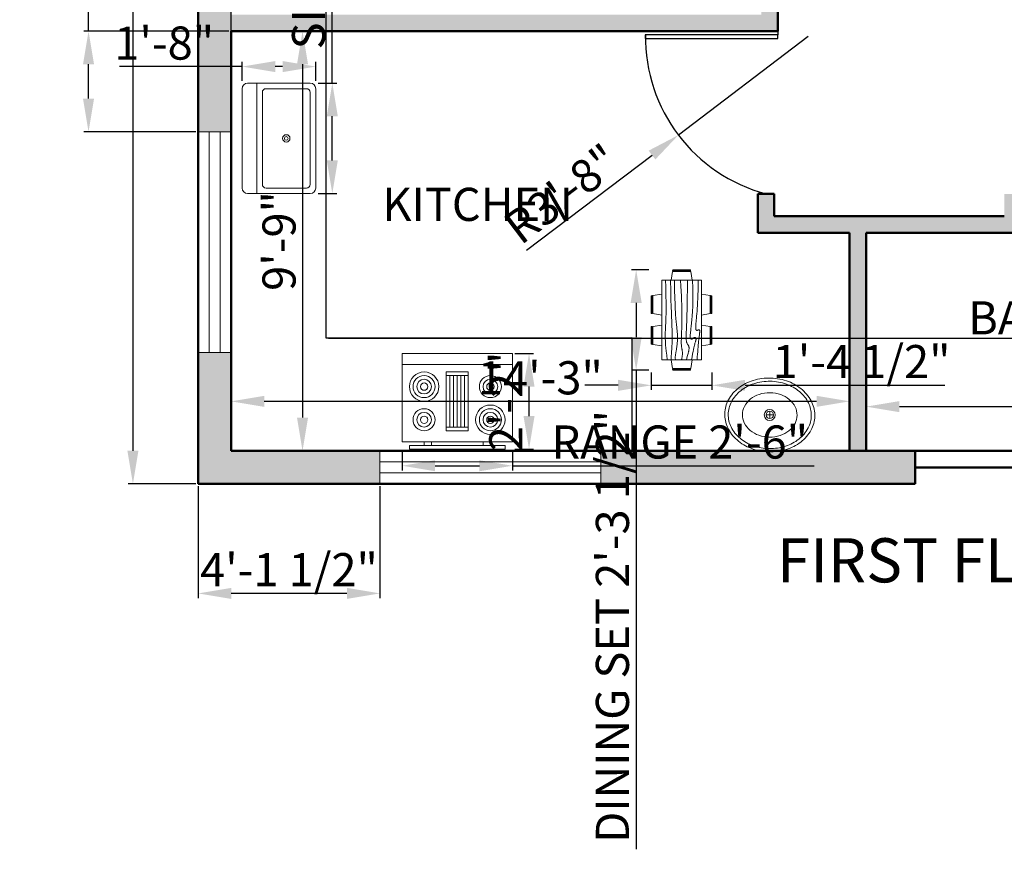
# Model space of a CAD drawing. Units: inches. Extents: x 875413 to 876020, y 447446 to 448210.
# Tile 1 of 8: x 875413 to 875681, y 447446 to 447671. Entities that reach past the tile are written whole.
import ezdxf

# ---------------------------------------------------------------- set-up
doc = ezdxf.new("R2010")
doc.units = ezdxf.units.IN
for name, color, linetype, lineweight in [('A-ANNO-DIMS', 2, 'Continuous', 13), ('A-ANNO-TEXT', 7, 'Continuous', 35), ('A-AREA-IDEN', 7, 'Continuous', 25), ('A-DOOR', 3, 'Continuous', 25), ('A-EQPM', 9, 'Continuous', 18), ('A-FLOR-CASE', 8, 'Continuous', 25), ('A-FLOR-FIXT', 9, 'Continuous', 18), ('A-FURN', 8, 'Continuous', 18), ('A-GLAZ', 4, 'Continuous', 20), ('A-WALL', 7, 'Continuous', 50)]:
    doc.layers.add(name, color=color, linetype=linetype, lineweight=lineweight)
doc.layers.add('A-WALL-PATT', color=18, linetype='Continuous', lineweight=13, true_color=0x000000)
doc.styles.get("Standard").update_dxf_attribs({"font": 'arial.ttf'})
doc.dimstyles.new('ISO-25', dxfattribs={"dimtxt": 9, "dimasz": 9, "dimexe": 1.25, "dimexo": 0.625, "dimtad": 1, "dimdec": 1, "dimrnd": 9, "dimlunit": 3, "dimtxsty": 'Standard', "dimcen": 2.5, "dimadec": 0, "dimazin": 0, "dimtfac": 1, "dimtdec": 1, "dimtmove": 0, "dimatfit": 3, "dimfxl": 1, "dimarcsym": 0})

# ---------------------------------------------------------------- blocks, each defined once
blk = doc.blocks.new('*D17')
at = {"layer": 'A-ANNO-DIMS', "color": 0, "lineweight": -2, "transparency": 16777216}
for p, q in [((875471.33, 447668.02), (875491.33, 447668.02)), ((875490.08, 447659.02), (875490.08, 447563.02)), ((875471.33, 447554.02), (875491.33, 447554.02))]:
    blk.add_line(p, q, dxfattribs=at)
at = {"layer": 'A-ANNO-DIMS', "color": 0, "transparency": 16777216}
for points in [[(875488.58, 447659.02), (875491.58, 447659.02), (875490.08, 447668.02)], [(875488.58, 447563.02), (875491.58, 447563.02), (875490.08, 447554.02)]]:
    blk.add_solid(points, dxfattribs=at)
at = {"layer": 'Defpoints', "color": 0, "transparency": 16777216}
for p in [(875470.7, 447668.02), (875470.7, 447554.02), (875490.08, 447554.02)]:
    blk.add_point(p, dxfattribs=at)
at = {"layer": 'A-ANNO-DIMS', "color": 0, "transparency": 16777216, "insert": (875484.86, 447611.02), "char_height": 9, "attachment_point": 5, "rotation": 90}
blk.add_mtext('9\'-9"', dxfattribs=at)
blk = doc.blocks.new('*D18')
at = {"layer": 'A-ANNO-DIMS', "color": 0, "lineweight": -2, "transparency": 16777216}
for p, q in [((875470.7, 447554.64), (875470.7, 447568.7)), ((875638.7, 447554.64), (875638.7, 447568.7)), ((875629.7, 447567.45), (875479.7, 447567.45))]:
    blk.add_line(p, q, dxfattribs=at)
at = {"layer": 'A-ANNO-DIMS', "color": 0, "transparency": 16777216}
for points in [[(875479.7, 447568.95), (875479.7, 447565.95), (875470.7, 447567.45)], [(875629.7, 447568.95), (875629.7, 447565.95), (875638.7, 447567.45)]]:
    blk.add_solid(points, dxfattribs=at)
at = {"layer": 'Defpoints', "color": 0, "transparency": 16777216}
for p in [(875470.7, 447567.45), (875470.7, 447554.02), (875638.7, 447554.02)]:
    blk.add_point(p, dxfattribs=at)
at = {"layer": 'A-ANNO-DIMS', "color": 0, "transparency": 16777216, "insert": (875554.7, 447572.68), "char_height": 9, "attachment_point": 5}
blk.add_mtext('14\'-3"', dxfattribs=at)
blk = doc.blocks.new('*D19')
at = {"layer": 'A-ANNO-DIMS', "color": 0, "lineweight": -2, "transparency": 16777216}
for p, q in [((875643.2, 447554.64), (875643.2, 447567.26)), ((875652.2, 447566.01), (875917.7, 447566.01)), ((875926.7, 447554.64), (875926.7, 447567.26))]:
    blk.add_line(p, q, dxfattribs=at)
at = {"layer": 'A-ANNO-DIMS', "color": 0, "transparency": 16777216}
for points in [[(875652.2, 447567.51), (875652.2, 447564.51), (875643.2, 447566.01)], [(875917.7, 447567.51), (875917.7, 447564.51), (875926.7, 447566.01)]]:
    blk.add_solid(points, dxfattribs=at)
at = {"layer": 'Defpoints', "color": 0, "transparency": 16777216}
for p in [(875926.7, 447566.01), (875643.2, 447554.02), (875926.7, 447554.02)]:
    blk.add_point(p, dxfattribs=at)
at = {"layer": 'A-ANNO-DIMS', "color": 0, "transparency": 16777216, "insert": (875784.95, 447571.15), "char_height": 9, "attachment_point": 5}
blk.add_mtext("24'", dxfattribs=at)
blk = doc.blocks.new('Dining Set - 36 x 72 in.')
for p, q in [((-22, 27.5), (-22.1562, 26.50042)), ((-22, 27.5), (-6, 27.5)), ((-5.8437, 26.49966), (-6, 27.5)), ((6, 27.5), (5.8438, 26.50042)), ((6, 27.5), (22, 27.5)), ((22.1563, 26.49966), (22, 27.5)), ((36, 18), (-36, 18)), ((-36, 18), (-36, -18)), ((-22.2343, 26.00059), (-23.4847, 17.99762)), ((-22.2304, 26), (-5.7608, 26)), ((-5.8416, 26.5), (-22.1534, 26.5)), ((-4.5152, 17.99762), (-5.7655, 25.99926)), ((5.7657, 26.00059), (4.5153, 17.99762)), ((5.7696, 26), (22.2392, 26)), ((22.1584, 26.5), (5.8466, 26.5)), ((23.4848, 17.99762), (22.2345, 25.99926)), ((36, -18), (36, 18)), ((-44.0006, 8.23428), (-35.9976, 9.48474)), ((44.0006, 8.23428), (35.9976, 9.48474)), ((-45.5, 8), (-44.5004, 8.15617)), ((-45.5, 8), (-45.5, -8)), ((-44.5, -8.15843), (-44.5, 8.15338)), ((-44, 8.23041), (-44, -8.23915)), ((44, 8.23041), (44, -8.23915)), ((44.5, -8.15843), (44.5, 8.15338)), ((45.5, 8), (44.5005, 8.15617)), ((45.5, 8), (45.5, -8)), ((-44.4997, -8.15631), (-45.5, -8)), ((-35.9976, -9.48476), (-43.9993, -8.2345)), ((35.9976, -9.48476), (43.9993, -8.2345)), ((44.4997, -8.15631), (45.5, -8)), ((-36, -18), (36, -18)), ((-22.2343, -26.0006), (-23.4847, -17.99762)), ((-22.2304, -26), (-5.7608, -26)), ((-22, -27.5), (-22.1562, -26.50044)), ((-5.8416, -26.5), (-22.1534, -26.5)), ((-5.8437, -26.49967), (-6, -27.5)), ((-4.5152, -17.99762), (-5.7655, -25.99928)), ((5.7657, -26.0006), (4.5153, -17.99762)), ((5.7696, -26), (22.2392, -26)), ((6, -27.5), (5.8438, -26.50044)), ((22.1584, -26.5), (5.8466, -26.5)), ((22.1563, -26.49967), (22, -27.5)), ((23.4848, -17.99762), (22.2345, -25.99928)), ((-22, -27.5), (-6, -27.5)), ((6, -27.5), (22, -27.5))]:
    blk.add_line(p, q)
for points in [[(-36, 15), (-31.1772, 14.97754), (-26.8079, 14.91406), (-22.8538, 14.81543), (-19.276, 14.6875), (-16.0362, 14.53613), (-13.0957, 14.36718), (-10.4159, 14.18652), (-7.9583, 14), (-5.6904, 13.81315), (-3.6035, 13.63021), (-1.6954, 13.45508), (0.0365, 13.29166), (1.5945, 13.14388), (2.9811, 13.01562), (4.1988, 12.9108), (5.25, 12.83333), (6.1393, 12.78613), (6.8802, 12.76823), (7.4883, 12.77767), (7.9792, 12.8125), (8.3685, 12.87077), (8.6719, 12.95052), (8.9049, 13.0498), (9.0833, 13.16666), (9.2205, 13.29899), (9.3216, 13.44401), (9.3895, 13.59879), (9.4271, 13.76041), (9.4373, 13.92594), (9.4232, 14.09245), (9.3875, 14.257), (9.3333, 14.41666), (9.2638, 14.56917), (9.1836, 14.71484), (9.0975, 14.85465), (9.0104, 14.98958), (8.9272, 15.1206), (8.8529, 15.2487), (8.7922, 15.37483), (8.75, 15.5), (8.7305, 15.62467), (8.7344, 15.74739), (8.7617, 15.86621), (8.8125, 15.97916), (8.8867, 16.08431), (8.9844, 16.17968), (9.1055, 16.26334), (9.25, 16.33333), (9.4189, 16.38802), (9.6172, 16.42708), (9.8506, 16.45052), (10.125, 16.45833), (10.4463, 16.45052), (10.8203, 16.42708), (11.2529, 16.38802), (11.75, 16.33333), (12.3184, 16.26318), (12.9694, 16.17838), (13.7151, 16.07991), (14.5677, 15.96875), (15.5395, 15.84586), (16.6426, 15.71224), (17.8893, 15.56884), (19.2917, 15.41666), (20.859, 15.25667), (22.5879, 15.08984), (24.4721, 14.91715), (26.5052, 14.73958), (28.6809, 14.5581), (30.9929, 14.3737), (33.4347, 14.18733), (36, 14)], [(-36, 10), (-28.9766, 10.14274), (-23.1725, 10.20442), (-18.4241, 10.19775), (-14.5677, 10.13541), (-11.4399, 10.03011), (-8.877, 9.89453), (-6.7154, 9.74137), (-4.7917, 9.58333), (-2.9698, 9.43082), (-1.2246, 9.28515), (0.4415, 9.14534), (2.026, 9.01041), (3.5266, 8.87939), (4.9408, 8.7513), (6.266, 8.62516), (7.5, 8.5), (8.6411, 8.37549), (9.6914, 8.2539), (10.6538, 8.13818), (11.5312, 8.03125), (12.3267, 7.93603), (13.043, 7.85547), (13.6831, 7.79248), (14.25, 7.75), (14.7471, 7.7303), (15.1797, 7.73307), (15.5537, 7.75732), (15.875, 7.80208), (16.1494, 7.86637), (16.3828, 7.94922), (16.5811, 8.04964), (16.75, 8.16666), (16.8944, 8.29915), (17.0143, 8.44531), (17.1089, 8.60319), (17.1771, 8.77083), (17.218, 8.94629), (17.2305, 9.1276), (17.2137, 9.31282), (17.1667, 9.5), (17.0895, 9.6875), (16.987, 9.875), (16.8649, 10.0625), (16.7292, 10.25), (16.5856, 10.4375), (16.4401, 10.625), (16.2985, 10.8125), (16.1667, 11), (16.05, 11.18733), (15.9518, 11.3737), (15.8752, 11.5581), (15.8229, 11.73958), (15.798, 11.91715), (15.8034, 12.08984), (15.842, 12.25667), (15.9167, 12.41666), (16.0295, 12.56836), (16.1784, 12.70833), (16.3605, 12.83268), (16.5729, 12.9375), (16.8127, 13.01888), (17.0768, 13.07291), (17.3625, 13.0957), (17.6667, 13.08333), (17.9894, 13.03312), (18.3418, 12.94726), (18.7382, 12.82918), (19.1927, 12.68229), (19.7195, 12.51001), (20.3327, 12.31575), (21.0465, 12.10294), (21.875, 11.875), (22.8357, 11.63354), (23.959, 11.37304), (25.2786, 11.08618), (26.8282, 10.76562), (28.6414, 10.40405), (30.752, 9.99414), (33.1936, 9.52856), (36, 9)], [(-36, 5.5), (-30.7157, 5.3348), (-26.069, 5.20963), (-21.9946, 5.11767), (-18.4271, 5.05208), (-15.3009, 5.00602), (-12.5508, 4.97265), (-10.1112, 4.94515), (-7.9167, 4.91666), (-5.909, 4.88167), (-4.0586, 4.83984), (-2.3429, 4.79215), (-0.7396, 4.73958), (0.7739, 4.6831), (2.22, 4.6237), (3.6213, 4.56233), (5, 4.5), (6.373, 4.43782), (7.7344, 4.3776), (9.0723, 4.32129), (10.375, 4.27083), (11.6309, 4.22819), (12.8281, 4.19531), (13.9551, 4.17415), (15, 4.16666), (15.954, 4.17448), (16.819, 4.19791), (17.6001, 4.23698), (18.3021, 4.29166), (18.9299, 4.36198), (19.4883, 4.44791), (19.9823, 4.54948), (20.4167, 4.66666), (20.7969, 4.79899), (21.1302, 4.94401), (21.4245, 5.09879), (21.6875, 5.26041), (21.9271, 5.42594), (22.1511, 5.59245), (22.3672, 5.757), (22.5834, 5.91666), (22.8065, 6.06868), (23.0404, 6.21093), (23.2879, 6.34147), (23.5521, 6.45833), (23.8358, 6.55957), (24.142, 6.64323), (24.4735, 6.70735), (24.8334, 6.75), (25.2235, 6.76969), (25.642, 6.76692), (26.0858, 6.74267), (26.5521, 6.69791), (27.0379, 6.63362), (27.5404, 6.55078), (28.0565, 6.45036), (28.5834, 6.33333), (29.1242, 6.19987), (29.7071, 6.04687), (30.3661, 5.87044), (31.1354, 5.66666), (32.0493, 5.43164), (33.142, 5.16146), (34.4475, 4.85221), (36, 4.5)], [(-36, -1), (-30.7915, -0.6591), (-26.0195, -0.38216), (-21.6519, -0.16284), (-17.6563, 0.00521), (-14.0005, 0.12833), (-10.6523, 0.21289), (-7.5796, 0.26522), (-4.75, 0.29166), (-2.134, 0.29793), (0.2878, 0.28711), (2.5317, 0.26163), (4.6146, 0.22396), (6.5529, 0.17651), (8.3633, 0.12174), (10.0623, 0.06209), (11.6667, 0), (13.1899, -0.06201), (14.6341, -0.1211), (15.9982, -0.17432), (17.2813, -0.21875), (18.4823, -0.25147), (19.6003, -0.26953), (20.6343, -0.27002), (21.5834, -0.25), (22.4481, -0.20768), (23.2357, -0.14584), (23.9549, -0.06836), (24.6146, 0.02083), (25.2235, 0.11784), (25.7904, 0.21875), (26.3241, 0.31966), (26.8334, 0.41666), (27.3265, 0.50618), (27.8099, 0.58593), (28.2894, 0.65397), (28.7709, 0.70833), (29.2601, 0.74707), (29.763, 0.76823), (30.2855, 0.76985), (30.8334, 0.75), (31.4088, 0.70784), (31.9994, 0.64713), (32.589, 0.57275), (33.1615, 0.48958), (33.7008, 0.4025), (34.1908, 0.3164), (34.6153, 0.23616), (34.9584, 0.16666), (35.2099, 0.11165), (35.3848, 0.07031), (35.504, 0.04069), (35.5886, 0.02083), (35.6594, 0.00879), (35.7377, 0.0026), (35.8442, 0.00032), (36, 0)], [(-36, -6.5), (-27.1843, -6.31267), (-20.084, -6.1263), (-14.469, -5.9419), (-10.1094, -5.76042), (-6.7752, -5.58285), (-4.2363, -5.41016), (-2.2629, -5.24333), (-0.625, -5.08334), (0.8708, -4.93099), (2.2715, -4.78646), (3.5872, -4.64974), (4.8281, -4.52084), (6.0046, -4.39974), (7.127, -4.28646), (8.2053, -4.18099), (9.25, -4.08334), (10.2705, -3.99382), (11.2734, -3.91407), (12.2647, -3.84603), (13.25, -3.79167), (14.2354, -3.75293), (15.2266, -3.73177), (16.2295, -3.73015), (17.25, -3.75), (18.2912, -3.79248), (19.3451, -3.85547), (20.4009, -3.93604), (21.4479, -4.03125), (22.4754, -4.13819), (23.4727, -4.25391), (24.4289, -4.37549), (25.3334, -4.5), (26.1785, -4.62492), (26.9694, -4.74935), (27.7145, -4.87281), (28.4219, -4.99479), (29.1, -5.11483), (29.7572, -5.23242), (30.4016, -5.34709), (31.0417, -5.45834), (31.6837, -5.56437), (32.3262, -5.65821), (32.9658, -5.73153), (33.599, -5.77604), (34.2224, -5.78345), (34.8327, -5.74545), (35.4264, -5.65373), (36, -5.5)], [(-36, -10), (-26.4022, -9.81299), (-18.4675, -9.62891), (-11.9839, -9.45069), (-6.7396, -9.28125), (-2.5226, -9.12354), (0.8789, -8.98047), (3.6769, -8.85498), (6.0833, -8.75), (8.2767, -8.66765), (10.3021, -8.60677), (12.1712, -8.56543), (13.8958, -8.54167), (15.4876, -8.53353), (16.9583, -8.53907), (18.3197, -8.55632), (19.5834, -8.58334), (20.7616, -8.61841), (21.8685, -8.66081), (22.9188, -8.71004), (23.9271, -8.76563), (24.9081, -8.82707), (25.8763, -8.89388), (26.8465, -8.96558), (27.8334, -9.04167), (28.8474, -9.12118), (29.8828, -9.20117), (30.93, -9.27824), (31.9792, -9.34896), (33.0205, -9.40991), (34.0443, -9.45768), (35.0407, -9.48885), (36, -9.5)], [(-36, -14.5), (-30.0881, -14.33513), (-25.0332, -14.21224), (-20.7312, -14.12647), (-17.0781, -14.07292), (-13.97, -14.04671), (-11.3027, -14.04297), (-8.9724, -14.05681), (-6.875, -14.08334), (-4.9224, -14.11833), (-3.0905, -14.16016), (-1.3709, -14.20785), (0.2448, -14.26042), (1.7647, -14.3169), (3.1973, -14.3763), (4.5507, -14.43767), (5.8333, -14.5), (7.0554, -14.5621), (8.235, -14.62175), (9.3922, -14.67652), (10.5469, -14.72396), (11.7192, -14.76164), (12.929, -14.78711), (14.1965, -14.79794), (15.5417, -14.79167), (16.9933, -14.76424), (18.6152, -14.70508), (20.4804, -14.60197), (22.6615, -14.44271), (25.2312, -14.21509), (28.2624, -13.9069), (31.8277, -13.50594), (36, -13)]]:
    blk.add_lwpolyline(points)
blk = doc.blocks.new('Range-Oven - 30 in top')
for p, q in [((0, -3), (30, -3)), ((12, -6), (18, -6)), ((13, -20), (13, -6)), ((14, -6), (14, -20)), ((15, -20), (15, -6)), ((16, -6), (16, -20)), ((17, -20), (17, -6)), ((18, -20), (12, -20)), ((6, -24), (6, -25)), ((8, -25), (8, -24)), ((22, -25), (22, -24)), ((24, -24), (24, -25))]:
    blk.add_line(p, q)
for points in [[(0, -24), (0, 0), (30, 0), (30, -24)], [(12, -21), (12, -5), (18, -5), (18, -21)], [(2, -26), (2, -25), (28, -25), (28, -26)]]:
    blk.add_lwpolyline(points, close=True)
for centre, radius in [((6, -9), 4), ((6, -9), 3), ((6, -9), 2), ((6, -9), 1), ((24, -9), 3), ((24, -9), 2), ((24, -9), 1), ((6, -18), 3), ((6, -18), 2), ((24, -18), 4), ((24, -18), 3), ((24, -18), 2), ((6, -18), 1), ((24, -18), 1)]:
    blk.add_circle(centre, radius)
blk = doc.blocks.new('Sink-single - 30 in top')
blk.add_line((-15, -3.999996), (15, -3.999996))
for points in [[(-13.5, 0), (13.5, 0)], [(-15, -18.499996), (-15, -1.5)], [(15, -1.5), (15, -18.499996)], [(-13.5, -17.499996), (-13.5, -6.499996)], [(-12.5, -5.499996), (12.5, -5.499996)], [(13.5, -6.499996), (13.5, -17.499996)], [(12.5, -18.499996), (-12.5, -18.499996)], [(13.5, -19.999996), (-13.5, -19.999996)]]:
    blk.add_lwpolyline(points)
for radius in [1, 0.5]:
    blk.add_circle((0, -11.999996), radius)
for centre, radius, start, end in [((-13.5, -1.5), 1.5, 90, 180), ((13.5, -1.5), 1.5, 0, 90), ((-12.5, -6.499996), 1, 90, 180), ((12.5, -6.499996), 1, 0, 90), ((-13.5, -18.499996), 1.5, 180, 270), ((-12.5, -17.499996), 1, 180, 270), ((12.5, -17.499996), 1, 270, 0), ((13.5, -18.499996), 1.5, 270, 0)]:
    blk.add_arc(centre, radius, start, end)
blk = doc.blocks.new('Sink - Oval top')
for p, q in [((-1, 0), (1, 0)), ((0, 1), (0, -1))]:
    blk.add_line(p, q)
for points in [[(-12.23, 0.39, 0.117634), (-11.46, -3.36, 0.104469), (-8.88, -6.8, 0.090016), (-5.08, -9.07, 0.08192), (-0.32, -10.02, 0.08192), (4.49, -9.38, 0.090016), (8.42, -7.36, 0.104469), (11.22, -4.09, 0.117634), (12.23, -0.39, 0.117634), (11.46, 3.36, 0.104469), (8.88, 6.8, 0.090016), (5.08, 9.07, 0.08192), (0.32, 10.02, 0.08192), (-4.49, 9.38, 0.090016), (-8.42, 7.36, 0.104469), (-11.22, 4.09, 0.117634)], [(-11.29, 0.16, 0.118622), (-10.52, -3.25, 0.104678), (-8.07, -6.36, 0.089562), (-4.54, -8.37, 0.081185), (-0.13, -9.15, 0.081185), (4.3, -8.49, 0.089562), (7.89, -6.58, 0.104678), (10.42, -3.55, 0.118622), (11.29, -0.16, 0.118622), (10.52, 3.25, 0.104678), (8.07, 6.36, 0.089562), (4.54, 8.37, 0.081185), (0.13, 9.15, 0.081185), (-4.3, 8.49, 0.089562), (-7.89, 6.58, 0.104678), (-10.42, 3.55, 0.118622)], [(-7.42, 0.08, 0.118283), (-6.91, -2.17, 0.104607), (-5.29, -4.21, 0.089718), (-2.97, -5.53, 0.081436), (-0.07, -6.04, 0.081436), (2.84, -5.59, 0.089718), (5.2, -4.33, 0.104607), (6.86, -2.32, 0.118283), (7.42, -0.08, 0.118283), (6.91, 2.17, 0.104607), (5.29, 4.21, 0.089718), (2.97, 5.53, 0.081436), (0.07, 6.04, 0.081436), (-2.84, 5.59, 0.089718), (-5.2, 4.33, 0.104607), (-6.86, 2.32, 0.118283)]]:
    blk.add_lwpolyline(points, format="xyb", close=True)
for radius in [1.5, 1]:
    blk.add_circle((0, 0), radius)
blk = doc.blocks.new('*D38')
at = {"layer": 'A-ANNO-DIMS', "color": 0, "lineweight": -2, "transparency": 16777216}
for p, q in [((875461.08, 448079.02), (875442.76, 448079.02)), ((875444.01, 448070.02), (875444.01, 447554.02)), ((875461.08, 447545.02), (875442.76, 447545.02))]:
    blk.add_line(p, q, dxfattribs=at)
at = {"layer": 'A-ANNO-DIMS', "color": 0, "transparency": 16777216}
for points in [[(875442.51, 448070.02), (875445.51, 448070.02), (875444.01, 448079.02)], [(875442.51, 447554.02), (875445.51, 447554.02), (875444.01, 447545.02)]]:
    blk.add_solid(points, dxfattribs=at)
at = {"layer": 'Defpoints', "color": 0, "transparency": 16777216}
for p in [(875461.7, 448079.02), (875444.01, 447545.02), (875461.7, 447545.02)]:
    blk.add_point(p, dxfattribs=at)
at = {"layer": 'A-ANNO-DIMS', "color": 0, "transparency": 16777216, "insert": (875438.78, 447812.02), "char_height": 9, "attachment_point": 5, "rotation": 90}
blk.add_mtext('44\'-3"', dxfattribs=at)
blk = doc.blocks.new('WIN-60IN')
for p, q in [((0, 9), (0, 0)), ((60, 9), (60, 0)), ((60, 6), (0, 6)), ((60, 3), (0, 3))]:
    blk.add_line(p, q)
blk = doc.blocks.new('*D55')
at = {"layer": 'A-ANNO-DIMS', "color": 0, "lineweight": -2, "transparency": 16777216}
for p, q in [((875584.18, 447603.19), (875579.46, 447603.19)), ((875580.71, 447594.19), (875580.71, 447584.89)), ((875584.18, 447575.89), (875579.46, 447575.89)), ((875580.71, 447575.89), (875580.71, 447445.75))]:
    blk.add_line(p, q, dxfattribs=at)
at = {"layer": 'A-ANNO-DIMS', "color": 0, "transparency": 16777216}
for points in [[(875579.21, 447594.19), (875582.21, 447594.19), (875580.71, 447603.19)], [(875579.21, 447584.89), (875582.21, 447584.89), (875580.71, 447575.89)]]:
    blk.add_solid(points, dxfattribs=at)
at = {"layer": 'Defpoints', "color": 0, "transparency": 16777216}
for p in [(875584.8, 447603.19), (875580.71, 447575.89), (875584.8, 447575.89)]:
    blk.add_point(p, dxfattribs=at)
at = {"layer": 'A-ANNO-DIMS', "color": 0, "transparency": 16777216, "insert": (875575.42, 447506.32), "char_height": 9, "attachment_point": 5, "rotation": 90}
blk.add_mtext('DINING SET 2\'-3 1/2"', dxfattribs=at)
blk = doc.blocks.new('*D56')
at = {"layer": 'A-ANNO-DIMS', "color": 0, "lineweight": -2, "transparency": 16777216}
for p, q in [((875584.8, 447575.27), (875584.8, 447570.55)), ((875601.3, 447575.27), (875601.3, 447570.55)), ((875575.8, 447571.8), (875566.8, 447571.8)), ((875584.8, 447571.8), (875601.3, 447571.8)), ((875610.3, 447571.8), (875664.6, 447571.8))]:
    blk.add_line(p, q, dxfattribs=at)
at = {"layer": 'A-ANNO-DIMS', "color": 0, "transparency": 16777216}
for points in [[(875575.8, 447573.3), (875575.8, 447570.3), (875584.8, 447571.8)], [(875610.3, 447573.3), (875610.3, 447570.3), (875601.3, 447571.8)]]:
    blk.add_solid(points, dxfattribs=at)
at = {"layer": 'Defpoints', "color": 0, "transparency": 16777216}
for p in [(875584.8, 447575.89), (875601.3, 447575.89), (875601.3, 447571.8)]:
    blk.add_point(p, dxfattribs=at)
at = {"layer": 'A-ANNO-DIMS', "color": 0, "transparency": 16777216, "insert": (875641.95, 447577.08), "char_height": 9, "attachment_point": 5}
blk.add_mtext('1\'-4 1/2"', dxfattribs=at)
blk = doc.blocks.new('*D63')
at = {"layer": 'A-ANNO-DIMS', "color": 0, "lineweight": -2, "transparency": 16777216}
for p, q in [((875517.11, 447553.83), (875517.11, 447548.7)), ((875547.11, 447553.83), (875547.11, 447548.7)), ((875526.11, 447549.95), (875538.11, 447549.95)), ((875547.11, 447549.95), (875629.02, 447549.95))]:
    blk.add_line(p, q, dxfattribs=at)
at = {"layer": 'A-ANNO-DIMS', "color": 0, "transparency": 16777216}
for points in [[(875526.11, 447551.45), (875526.11, 447548.45), (875517.11, 447549.95)], [(875538.11, 447551.45), (875538.11, 447548.45), (875547.11, 447549.95)]]:
    blk.add_solid(points, dxfattribs=at)
at = {"layer": 'Defpoints', "color": 0, "transparency": 16777216}
for p in [(875517.11, 447554.45), (875547.11, 447554.45), (875547.11, 447549.95)]:
    blk.add_point(p, dxfattribs=at)
at = {"layer": 'A-ANNO-DIMS', "color": 0, "transparency": 16777216, "insert": (875592.57, 447555.23), "char_height": 9, "attachment_point": 5}
blk.add_mtext('RANGE 2\'-6"', dxfattribs=at)
blk = doc.blocks.new('*D64')
at = {"layer": 'A-ANNO-DIMS', "color": 0, "lineweight": -2, "transparency": 16777216}
for p, q in [((875547.74, 447580.45), (875552.86, 447580.45)), ((875551.61, 447563.45), (875551.61, 447571.45)), ((875547.74, 447554.45), (875552.86, 447554.45))]:
    blk.add_line(p, q, dxfattribs=at)
at = {"layer": 'A-ANNO-DIMS', "color": 0, "transparency": 16777216}
for points in [[(875550.11, 447571.45), (875553.11, 447571.45), (875551.61, 447580.45)], [(875550.11, 447563.45), (875553.11, 447563.45), (875551.61, 447554.45)]]:
    blk.add_solid(points, dxfattribs=at)
at = {"layer": 'Defpoints', "color": 0, "transparency": 16777216}
for p in [(875547.11, 447580.45), (875551.61, 447580.45), (875547.11, 447554.45)]:
    blk.add_point(p, dxfattribs=at)
at = {"layer": 'A-ANNO-DIMS', "color": 0, "transparency": 16777216, "insert": (875546.47, 447567.45), "char_height": 9, "attachment_point": 5, "rotation": 90}
blk.add_mtext('2\'-2"', dxfattribs=at)
blk = doc.blocks.new('*D65')
at = {"layer": 'A-ANNO-DIMS', "color": 0, "lineweight": -2, "transparency": 16777216}
for p, q in [((875498.17, 447653.89), (875498.17, 447720.86)), ((875494.3, 447653.89), (875499.42, 447653.89)), ((875498.17, 447632.89), (875498.17, 447644.89)), ((875494.3, 447623.89), (875499.42, 447623.89))]:
    blk.add_line(p, q, dxfattribs=at)
at = {"layer": 'A-ANNO-DIMS', "color": 0, "transparency": 16777216}
for points in [[(875496.67, 447644.89), (875499.67, 447644.89), (875498.17, 447653.89)], [(875496.67, 447632.89), (875499.67, 447632.89), (875498.17, 447623.89)]]:
    blk.add_solid(points, dxfattribs=at)
at = {"layer": 'Defpoints', "color": 0, "transparency": 16777216}
for p in [(875493.67, 447653.89), (875498.17, 447653.89), (875493.67, 447623.89)]:
    blk.add_point(p, dxfattribs=at)
at = {"layer": 'A-ANNO-DIMS', "color": 0, "transparency": 16777216, "insert": (875492.89, 447691.87), "char_height": 9, "attachment_point": 5, "rotation": 90}
blk.add_mtext('SINK 2\'-6"', dxfattribs=at)
blk = doc.blocks.new('*D66')
at = {"layer": 'A-ANNO-DIMS', "color": 0, "lineweight": -2, "transparency": 16777216}
for p, q in [((875473.67, 447654.51), (875473.67, 447659.64)), ((875493.67, 447654.51), (875493.67, 447659.64)), ((875473.67, 447658.39), (875440.34, 447658.39)), ((875484.67, 447658.39), (875482.67, 447658.39))]:
    blk.add_line(p, q, dxfattribs=at)
at = {"layer": 'A-ANNO-DIMS', "color": 0, "transparency": 16777216}
for points in [[(875482.67, 447659.89), (875482.67, 447656.89), (875473.67, 447658.39)], [(875484.67, 447659.89), (875484.67, 447656.89), (875493.67, 447658.39)]]:
    blk.add_solid(points, dxfattribs=at)
at = {"layer": 'Defpoints', "color": 0, "transparency": 16777216}
for p in [(875473.67, 447658.39), (875473.67, 447653.89), (875493.67, 447653.89)]:
    blk.add_point(p, dxfattribs=at)
at = {"layer": 'A-ANNO-DIMS', "color": 0, "transparency": 16777216, "insert": (875452.51, 447663.61), "char_height": 9, "attachment_point": 5}
blk.add_mtext('1\'-8"', dxfattribs=at)
blk = doc.blocks.new('*D73')
at = {"layer": 'A-ANNO-DIMS', "color": 0, "lineweight": -2, "transparency": 16777216}
for p, q in [((875431.95, 447668.02), (875431.95, 447723.32)), ((875470.08, 447668.02), (875430.7, 447668.02)), ((875431.95, 447649.7), (875431.95, 447659.02)), ((875461.08, 447640.7), (875430.7, 447640.7))]:
    blk.add_line(p, q, dxfattribs=at)
at = {"layer": 'A-ANNO-DIMS', "color": 0, "transparency": 16777216}
for points in [[(875430.45, 447659.02), (875433.45, 447659.02), (875431.95, 447668.02)], [(875430.45, 447649.7), (875433.45, 447649.7), (875431.95, 447640.7)]]:
    blk.add_solid(points, dxfattribs=at)
at = {"layer": 'Defpoints', "color": 0, "transparency": 16777216}
for p in [(875431.95, 447668.02), (875470.7, 447668.02), (875461.7, 447640.7)]:
    blk.add_point(p, dxfattribs=at)
at = {"layer": 'A-ANNO-DIMS', "color": 0, "transparency": 16777216, "insert": (875426.67, 447700.17), "char_height": 9, "attachment_point": 5, "rotation": 90}
blk.add_mtext('2\'-3 1/2"', dxfattribs=at)
blk = doc.blocks.new('*D74')
at = {"layer": 'A-ANNO-DIMS', "color": 0, "lineweight": -2, "transparency": 16777216}
for p, q in [((875461.7, 447544.39), (875461.7, 447514.02)), ((875511.12, 447544.39), (875511.12, 447514.02)), ((875502.12, 447515.27), (875470.7, 447515.27))]:
    blk.add_line(p, q, dxfattribs=at)
at = {"layer": 'A-ANNO-DIMS', "color": 0, "transparency": 16777216}
for points in [[(875470.7, 447516.77), (875470.7, 447513.77), (875461.7, 447515.27)], [(875502.12, 447516.77), (875502.12, 447513.77), (875511.12, 447515.27)]]:
    blk.add_solid(points, dxfattribs=at)
at = {"layer": 'Defpoints', "color": 0, "transparency": 16777216}
for p in [(875461.7, 447545.02), (875511.12, 447545.02), (875461.7, 447515.27)]:
    blk.add_point(p, dxfattribs=at)
at = {"layer": 'A-ANNO-DIMS', "color": 0, "transparency": 16777216, "insert": (875486.41, 447520.55), "char_height": 9, "attachment_point": 5}
blk.add_mtext('4\'-1 1/2"', dxfattribs=at)
blk = doc.blocks.new('*D82')
at = {"layer": 'A-ANNO-DIMS', "color": 0, "lineweight": -2, "transparency": 16777216}
for p, q in [((875470.7, 447554.64), (875470.7, 448110.02)), ((875487.52, 448108.77), (875479.7, 448108.77)), ((875496.52, 447585.21), (875496.52, 448110.02))]:
    blk.add_line(p, q, dxfattribs=at)
at = {"layer": 'A-ANNO-DIMS', "color": 0, "transparency": 16777216}
for points in [[(875479.7, 448110.27), (875479.7, 448107.27), (875470.7, 448108.77)], [(875487.52, 448110.27), (875487.52, 448107.27), (875496.52, 448108.77)]]:
    blk.add_solid(points, dxfattribs=at)
at = {"layer": 'Defpoints', "color": 0, "transparency": 16777216}
for p in [(875470.7, 448108.77), (875496.52, 447584.59), (875470.7, 447554.02)]:
    blk.add_point(p, dxfattribs=at)
at = {"layer": 'A-ANNO-DIMS', "color": 0, "transparency": 16777216, "insert": (875483.61, 448113.91), "char_height": 9, "attachment_point": 5}
blk.add_mtext('2\'-2"', dxfattribs=at)
blk = doc.blocks.new('*D83')
at = {"layer": 'A-ANNO-DIMS', "color": 0, "lineweight": -2, "transparency": 16777216}
for p, q in [((875497.15, 447584.59), (875966.7, 447584.59)), ((875965.45, 447575.59), (875965.45, 447563.02)), ((875471.33, 447554.02), (875966.7, 447554.02)), ((875965.45, 447554.02), (875965.45, 447498.72))]:
    blk.add_line(p, q, dxfattribs=at)
at = {"layer": 'A-ANNO-DIMS', "color": 0, "transparency": 16777216}
for points in [[(875963.95, 447575.59), (875966.95, 447575.59), (875965.45, 447584.59)], [(875963.95, 447563.02), (875966.95, 447563.02), (875965.45, 447554.02)]]:
    blk.add_solid(points, dxfattribs=at)
at = {"layer": 'Defpoints', "color": 0, "transparency": 16777216}
for p in [(875496.52, 447584.59), (875470.7, 447554.02), (875965.45, 447554.02)]:
    blk.add_point(p, dxfattribs=at)
at = {"layer": 'A-ANNO-DIMS', "color": 0, "transparency": 16777216, "insert": (875960.17, 447521.87), "char_height": 9, "attachment_point": 5, "rotation": 90}
blk.add_mtext('2\'-6 1/2"', dxfattribs=at)
blk = doc.blocks.new('*D92')
at = {"layer": 'A-ANNO-DIMS', "color": 0, "lineweight": -2, "transparency": 16777216}
for p, q in [((875627.42, 447666.52), (875592.19, 447639.79)), ((875550.92, 447608.5), (875585.02, 447634.36))]:
    blk.add_line(p, q, dxfattribs=at)
at = {"layer": 'A-ANNO-DIMS', "color": 0, "transparency": 16777216}
blk.add_solid([(875584.11, 447635.55), (875585.92, 447633.16), (875592.19, 447639.79)], dxfattribs=at)
at = {"layer": 'Defpoints', "color": 0, "transparency": 16777216}
for p in [(875627.42, 447666.52), (875592.19, 447639.79)]:
    blk.add_point(p, dxfattribs=at)
at = {"layer": 'A-ANNO-DIMS', "color": 0, "transparency": 16777216, "insert": (875561.23, 447622.87), "char_height": 9, "attachment_point": 5, "rotation": 37.1774}
blk.add_mtext('R3\'-8"', dxfattribs=at)

msp = doc.modelspace()

# ---------------------------------------------------------------- hatches: boundary and pattern name
at = {"layer": 'A-WALL-PATT'}
h = msp.add_hatch(color=256, dxfattribs=at)
h.dxf.hatch_style = 1
h.paths.add_polyline_path([(875470.7, 447985.13), (875461.7, 447985.13), (875461.7, 447865.29), (875470.7, 447865.29), (875470.7, 447881.02), (875566.7, 447881.02), (875566.7, 447797.02), (875571.2, 447797.02), (875571.2, 447885.52), (875571.2, 447921.52), (875603.29, 447921.52), (875603.29, 447926.02), (875501.27, 447926.02), (875501.27, 447921.52), (875566.7, 447921.52), (875566.7, 447885.52), (875470.7, 447885.52), (875470.7, 447921.52), (875470.7, 447926.02)])
h.paths.add_polyline_path([(875470.7, 448070.02), (875518.96, 448070.02), (875518.96, 448079.02), (875461.7, 448079.02), (875461.7, 448045.13), (875470.7, 448045.13)])
h.paths.add_polyline_path([(875819.9, 448079.02), (875578.96, 448079.02), (875578.96, 448070.02), (875638.7, 448070.02), (875638.7, 447921.52), (875643.2, 447921.52), (875643.2, 448070.02), (875763.2, 448070.02), (875763.2, 447921.52), (875767.7, 447921.52), (875767.7, 448070.02), (875819.9, 448070.02)])
h.paths.add_polyline_path([(875935.7, 447978.92), (875926.7, 447978.92), (875926.7, 447926.02), (875926.7, 447921.52), (875926.7, 447885.52), (875842.7, 447885.52), (875842.7, 447921.52), (875899.7, 447921.52), (875899.7, 447926.02), (875805.34, 447926.02), (875805.34, 447921.52), (875838.2, 447921.52), (875838.2, 447885.52), (875838.2, 447797.02), (875689.7, 447797.02), (875689.7, 447792.52), (875842.7, 447792.52), (875842.7, 447881.02), (875926.7, 447881.02), (875926.7, 447857.16), (875935.7, 447857.16)])
h.paths.add_polyline_path([(875935.7, 448079.02), (875879.9, 448079.02), (875879.9, 448070.02), (875926.7, 448070.02), (875926.7, 448038.92), (875935.7, 448038.92)])
h.paths.add_polyline_path([(875935.7, 447833.16), (875926.7, 447833.16), (875926.7, 447797.02), (875842.7, 447797.02), (875842.7, 447792.52), (875926.7, 447792.52), (875926.7, 447756.52), (875935.7, 447756.52)])
h.paths.add_polyline_path([(875935.7, 447732.52), (875926.7, 447732.52), (875926.7, 447692.75, -0.007222), (875926.81, 447692.41, -0.08192), (875927.45, 447687.6, -0.071798), (875926.7, 447683.4), (875926.7, 447672.52), (875808.63, 447672.52), (875808.63, 447668.02), (875926.7, 447668.02), (875926.7, 447663.19), (875935.7, 447663.19)])
h.paths.add_polyline_path([(875842.7, 447792.52), (875838.2, 447792.52), (875838.2, 447704.02), (875842.7, 447704.02)])
h.paths.add_polyline_path([(875470.7, 447792.52), (875619.2, 447792.52), (875619.2, 447797.02), (875470.7, 447797.02), (875470.7, 447841.29), (875461.7, 447841.29), (875461.7, 447764.71), (875470.7, 447764.71)])
h.paths.add_polyline_path([(875619.2, 447760.51), (875616.95, 447760.51, -0.018388), (875614.7, 447760.37), (875614.7, 447672.52), (875470.7, 447672.52), (875470.7, 447704.71), (875461.7, 447704.71), (875461.7, 447640.7), (875470.7, 447640.7), (875470.7, 447668.02), (875619.2, 447668.02)])
h.paths.add_polyline_path([(875511.12, 447554.02), (875470.7, 447554.02), (875470.7, 447580.7), (875461.7, 447580.7), (875461.7, 447545.02), (875511.12, 447545.02)])
h.paths.add_polyline_path([(875656.47, 447554.02), (875620.05, 447554.02, -0.057036), (875616.67, 447553.74, -0.040891), (875614.26, 447554.02), (875571.12, 447554.02), (875571.12, 447545.02), (875656.47, 447545.02)])
h.paths.add_polyline_path([(875643.2, 447613.27), (875685.21, 447613.27), (875685.21, 447617.77), (875685.21, 447623.8), (875680.71, 447623.8), (875680.71, 447617.77), (875618.23, 447617.77), (875618.23, 447623.8), (875613.73, 447623.8), (875613.73, 447617.77), (875613.73, 447613.27), (875638.7, 447613.27), (875638.7, 447554.02), (875643.2, 447554.02)])
h.paths.add_polyline_path([(875694.2, 447760.28), (875689.7, 447760.28), (875689.7, 447668.02), (875748.63, 447668.02), (875748.63, 447672.52), (875694.2, 447672.52)])

# ---------------------------------------------------------------- linework, layer by layer
at = {"layer": 'A-DOOR'}
for p, q in [((875619.2, 447667.02), (875583.2, 447667.02)), ((875583.2, 447667.02), (875583.2, 447666.02)), ((875619.2, 447668.02), (875619.2, 447667.02)), ((875619.2, 447666.02), (875619.2, 447667.02)), ((875583.2, 447666.02), (875619.2, 447666.02))]:
    msp.add_line(p, q, dxfattribs=at)
msp.add_arc((875627.42, 447666.52), 44.22, 179.3522, 255.0037, dxfattribs=at)
at = {"layer": 'A-FLOR-CASE'}
for p, q in [((875496.52, 447584.59), (875496.52, 447668.02)), ((875579.59, 447584.59), (875496.52, 447584.59)), ((875579.59, 447554.02), (875579.59, 447584.59))]:
    msp.add_line(p, q, dxfattribs=at)
at = {"layer": 'A-WALL'}
for p, q in [((875461.7, 448079.02), (875461.7, 447545.02)), ((875619.2, 447760.51), (875619.2, 447668.02)), ((875470.7, 447668.02), (875470.7, 447554.02)), ((875619.2, 447668.02), (875470.7, 447668.02)), ((875613.73, 447617.77), (875613.73, 447623.8)), ((875613.73, 447623.8), (875618.23, 447623.8)), ((875618.23, 447623.8), (875618.23, 447617.77)), ((875613.73, 447617.77), (875613.73, 447613.27)), ((875680.71, 447617.77), (875618.23, 447617.77)), ((875638.7, 447613.27), (875613.73, 447613.27)), ((875638.7, 447613.27), (875638.7, 447554.02)), ((875643.2, 447613.27), (875685.21, 447613.27)), ((875643.2, 447613.27), (875643.2, 447554.02)), ((875470.7, 447554.02), (875656.47, 447554.02)), ((875656.47, 447554.02), (875656.47, 447545.02)), ((875656.47, 447554.02), (875926.7, 447554.02)), ((875656.47, 447549.52), (875931.2, 447549.52)), ((875461.7, 447545.02), (875656.47, 447545.02))]:
    msp.add_line(p, q, dxfattribs=at)

# ---------------------------------------------------------------- block references
at = {"layer": 'A-EQPM'}
msp.add_blockref('Range-Oven - 30 in top', (875517.11, 447580.45), dxfattribs=at)
at = {"layer": 'A-FLOR-FIXT'}
for name, p, rotation in [('Sink-single - 30 in top', (875473.67, 447638.89), 90), ('Sink - Oval top', (875617, 447563.76), 180)]:
    msp.add_blockref(name, p, dxfattribs=dict(at, rotation=rotation))
at = {"layer": 'A-FURN', "xscale": 0.3, "yscale": 0.3, "rotation": 270}
msp.add_blockref('Dining Set - 36 x 72 in.', (875593.05, 447589.54), dxfattribs=at)
at = {"layer": 'A-GLAZ'}
for p, rotation in [((875461.7, 447640.7), 269.9999999998478), ((875571.12, 447554.02), 180)]:
    msp.add_blockref('WIN-60IN', p, dxfattribs=dict(at, rotation=rotation))

# ---------------------------------------------------------------- texts
at = {"layer": 'A-ANNO-TEXT', "insert": (875618.96, 447530.26), "char_height": 12, "attachment_point": 1}
msp.add_mtext_dynamic_manual_height_columns('FIRST FLOOR PLAN', width=417.4622, gutter_width=12.5, heights=[0], dxfattribs=at)
at = {"layer": 'A-AREA-IDEN', "char_height": 9, "attachment_point": 1}
for s, insert in [('KITCHEN', (875511.76, 447625.46)), ('BALCONY', (875670.9, 447594.63))]:
    msp.add_mtext_dynamic_manual_height_columns(s, width=100.7812, gutter_width=12.5, heights=[0], dxfattribs=dict(at, insert=insert))

# ---------------------------------------------------------------- dimensions: what is measured, and where the dimension line sits
at = {"layer": 'A-ANNO-DIMS'}
for base, p1, p2, override, picture, middle in [((875470.7, 448108.77), (875496.52, 447584.59), (875470.7, 447554.02), {"dimdec": 1, "dimlfac": 1, "dimrnd": 0, "dimzin": 1, "dimdsep": 46, "dimlunit": 4, "dimfrac": 2}, '*D82', (875483.61, 448113.91)), ((875601.3, 447571.8), (875584.8, 447575.89), (875601.3, 447575.89), {"dimdec": 1, "dimlfac": 1, "dimrnd": 0, "dimzin": 1, "dimdsep": 46, "dimlunit": 4, "dimfrac": 2}, '*D56', (875641.95, 447577.08)), ((875470.7, 447567.45), (875638.7, 447554.02), (875470.7, 447554.02), {"dimclrd": 0, "dimclre": 0, "dimclrt": 0}, '*D18', (875554.7, 447572.68)), ((875926.7, 447566.01), (875643.2, 447554.02), (875926.7, 447554.02), {"dimclrd": 0, "dimclre": 0, "dimclrt": 0}, '*D19', (875784.95, 447571.15)), ((875461.7, 447515.27), (875511.12, 447545.02), (875461.7, 447545.02), {"dimdec": 1, "dimlfac": 1, "dimrnd": 0, "dimzin": 1, "dimdsep": 46, "dimlunit": 4, "dimfrac": 2}, '*D74', (875486.41, 447520.55))]:
    dim = msp.add_linear_dim(base=base, p1=p1, p2=p2, dimstyle='ISO-25', override=override, dxfattribs=at)
    dim.commit()
    dim.dimension.update_dxf_attribs({"geometry": picture, "text_midpoint": middle})
for base, p1, p2, angle, override, picture, middle in [((875444.01, 447545.02), (875461.7, 448079.02), (875461.7, 447545.02), 90, {"dimclrd": 0, "dimclre": 0, "dimclrt": 0}, '*D38', (875438.78, 447812.02)), ((875431.95, 447668.02), (875461.7, 447640.7), (875470.7, 447668.02), 90, {"dimdec": 1, "dimlfac": 1, "dimrnd": 0, "dimzin": 1, "dimdsep": 46, "dimlunit": 4, "dimfrac": 2}, '*D73', (875426.67, 447700.17)), ((875473.67, 447658.39), (875493.67, 447653.89), (875473.67, 447653.89), 180, {"dimdec": 1, "dimlfac": 1, "dimrnd": 0, "dimzin": 1, "dimdsep": 46, "dimlunit": 4, "dimfrac": 2}, '*D66', (875452.51, 447663.61)), ((875490.08, 447554.02), (875470.7, 447668.02), (875470.7, 447554.02), 90, {"dimclrd": 0, "dimclre": 0, "dimclrt": 0}, '*D17', (875484.86, 447611.02)), ((875965.45, 447554.02), (875496.52, 447584.59), (875470.7, 447554.02), 90, {"dimdec": 1, "dimlfac": 1, "dimrnd": 0, "dimzin": 1, "dimdsep": 46, "dimlunit": 4, "dimfrac": 2}, '*D83', (875960.17, 447521.87)), ((875551.61, 447580.45), (875547.11, 447554.45), (875547.11, 447580.45), 90, {"dimdec": 1, "dimlfac": 1, "dimrnd": 0, "dimzin": 1, "dimdsep": 46, "dimlunit": 4, "dimfrac": 2}, '*D64', (875546.47, 447567.45))]:
    dim = msp.add_linear_dim(base=base, p1=p1, p2=p2, angle=angle, dimstyle='ISO-25', override=override, dxfattribs=at)
    dim.commit()
    dim.dimension.update_dxf_attribs({"geometry": picture, "text_midpoint": middle})
for base, p1, p2, angle, text, picture, middle in [((875498.17, 447653.89), (875493.67, 447623.89), (875493.67, 447653.89), 90, 'SINK <>', '*D65', (875492.89, 447691.87)), ((875580.71, 447575.89), (875584.8, 447603.19), (875584.8, 447575.89), 270, 'DINING SET <>', '*D55', (875575.42, 447506.32))]:
    dim = msp.add_linear_dim(base=base, p1=p1, p2=p2, angle=angle, text=text, dimstyle='ISO-25', override={"dimdec": 1, "dimlfac": 1, "dimrnd": 0, "dimzin": 1, "dimdsep": 46, "dimlunit": 4, "dimfrac": 2}, dxfattribs=at)
    dim.commit()
    dim.dimension.update_dxf_attribs({"geometry": picture, "text_midpoint": middle})
dim = msp.add_radius_dim(center=(875627.42, 447666.52), mpoint=(875592.19, 447639.79), dimstyle='ISO-25', override={"dimdec": 1, "dimlfac": 1, "dimrnd": 0, "dimzin": 1, "dimdsep": 46, "dimlunit": 4, "dimfrac": 2}, dxfattribs=at)
dim.commit()
dim.dimension.update_dxf_attribs({"geometry": '*D92', "text_midpoint": (875561.23, 447622.87)})
dim = msp.add_linear_dim(base=(875547.11, 447549.95), p1=(875517.11, 447554.45), p2=(875547.11, 447554.45), text='RANGE <>', dimstyle='ISO-25', override={"dimdec": 1, "dimlfac": 1, "dimrnd": 0, "dimzin": 1, "dimdsep": 46, "dimlunit": 4, "dimfrac": 2}, dxfattribs=at)
dim.commit()
dim.dimension.update_dxf_attribs({"geometry": '*D63', "text_midpoint": (875592.57, 447555.23)})

doc.saveas('drawing.dxf')
